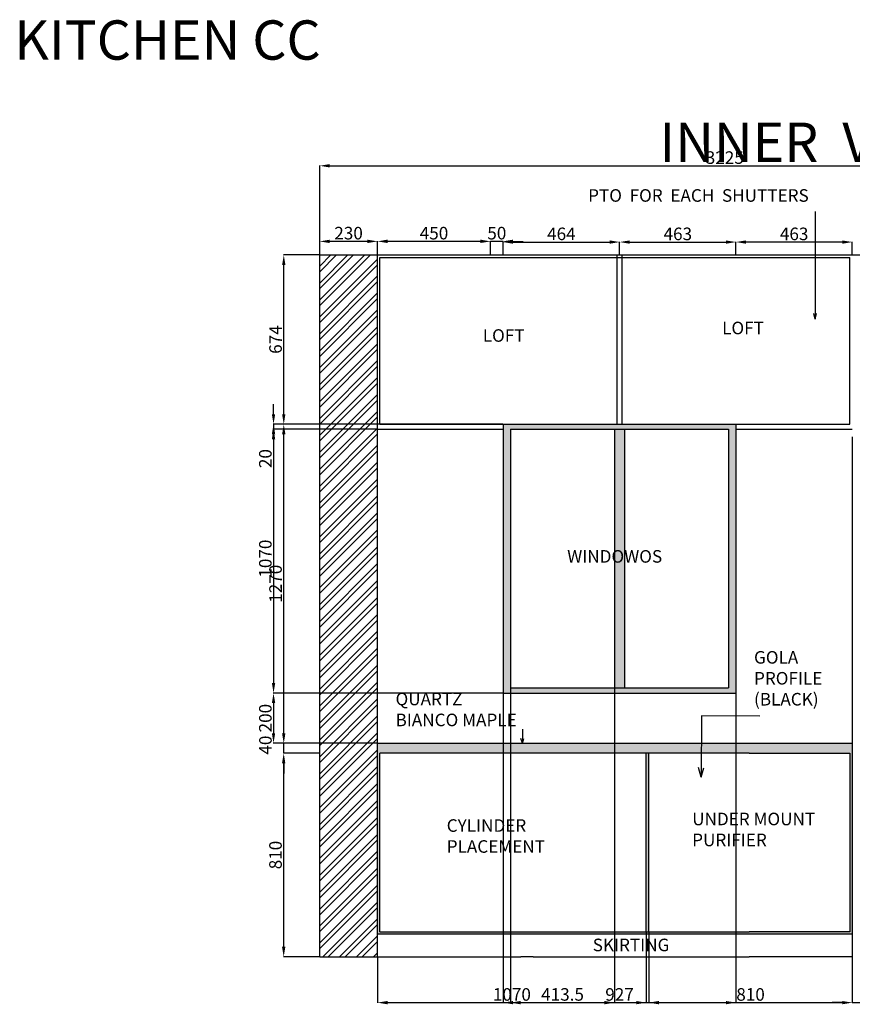
# Model space of a CAD drawing. Units: millimetres. Extents: x 144895 to 155057, y -2833 to 1092.
# Tile 3 of 4: x 148719 to 152033, y -2827 to 1092. Entities that reach past the tile are written whole.
import ezdxf

# ---------------------------------------------------------------- set-up
doc = ezdxf.new("R2010")
doc.units = ezdxf.units.MM
for name, color, linetype, lineweight in [('A-ANNO-DIMS', 2, 'Continuous', 18), ('A-ANNO-TEXT', 7, 'Continuous', 18), ('A-ELEV', 7, 'Continuous', 25), ('A-ELEV-PATT', 252, 'Continuous', 13), ('A-WALL-PATT', 8, 'Continuous', 13)]:
    doc.layers.add(name, color=color, linetype=linetype, lineweight=lineweight)
doc.styles.get("Standard").update_dxf_attribs({"font": 'arial.ttf'})
doc.dimstyles.new('ISO-25', dxfattribs={"dimtxt": 50, "dimasz": 40, "dimexe": 1.25, "dimexo": 0.625, "dimtad": 1, "dimtxsty": 'Standard', "dimcen": 2.5, "dimadec": 0, "dimazin": 0, "dimtfac": 1, "dimtmove": 0, "dimatfit": 3, "dimfxl": 1, "dimarcsym": 0})

# ---------------------------------------------------------------- blocks, each defined once
blk = doc.blocks.new('*D40')
at = {"layer": 'A-ANNO-DIMS', "color": 0, "lineweight": -2, "transparency": 16777216}
for p, q in [((149912.6, -1827.9), (149768.7, -1827.9)), ((149770, -2597.9), (149770, -1867.9)), ((149912.6, -2637.9), (149768.7, -2637.9))]:
    blk.add_line(p, q, dxfattribs=at)
at = {"layer": 'A-ANNO-DIMS', "color": 0, "transparency": 16777216}
for points in [[(149763.3, -1867.9), (149776.6, -1867.9), (149770, -1827.9)], [(149763.3, -2597.9), (149776.6, -2597.9), (149770, -2637.9)]]:
    blk.add_solid(points, dxfattribs=at)
at = {"layer": 'Defpoints', "color": 0, "transparency": 16777216}
for p in [(149770, -1827.9), (149913.2, -1827.9), (149913.2, -2637.9)]:
    blk.add_point(p, dxfattribs=at)
at = {"layer": 'A-ANNO-DIMS', "color": 0, "transparency": 16777216, "insert": (149743.8, -2232.9), "char_height": 50, "attachment_point": 5, "rotation": 90}
blk.add_mtext('810', dxfattribs=at)
blk = doc.blocks.new('*D32')
at = {"layer": 'A-ANNO-DIMS', "color": 0, "lineweight": -2, "transparency": 16777216}
for p, q in [((149770, -1747.9), (149770, -1707.9)), ((149912.6, -1787.9), (149768.7, -1787.9)), ((149770, -1827.9), (149770, -1787.9)), ((149912.6, -1827.9), (149768.7, -1827.9)), ((149770, -1867.9), (149770, -1907.9))]:
    blk.add_line(p, q, dxfattribs=at)
at = {"layer": 'A-ANNO-DIMS', "color": 0, "transparency": 16777216}
for points in [[(149763.3, -1747.9), (149776.6, -1747.9), (149770, -1787.9)], [(149763.3, -1867.9), (149776.6, -1867.9), (149770, -1827.9)]]:
    blk.add_solid(points, dxfattribs=at)
at = {"layer": 'Defpoints', "color": 0, "transparency": 16777216}
for p in [(149770, -1787.9), (149913.2, -1787.9), (149913.2, -1827.9)]:
    blk.add_point(p, dxfattribs=at)
at = {"layer": 'A-ANNO-DIMS', "color": 0, "transparency": 16777216, "insert": (149703.8, -1795.3), "char_height": 50, "attachment_point": 5, "rotation": 90}
blk.add_mtext('40', dxfattribs=at)
blk = doc.blocks.new('*D34')
at = {"layer": 'A-ANNO-DIMS', "color": 0, "lineweight": -2, "ltscale": 20, "transparency": 16777216}
for p, q in [((150143.2, 156.7), (150143.2, 211.4)), ((150553.2, 210.1), (150183.2, 210.1)), ((150593.2, 156.7), (150593.2, 211.4))]:
    blk.add_line(p, q, dxfattribs=at)
at = {"layer": 'A-ANNO-DIMS', "color": 0, "ltscale": 20, "transparency": 16777216}
for points in [[(150183.2, 216.8), (150183.2, 203.5), (150143.2, 210.1)], [(150553.2, 216.8), (150553.2, 203.5), (150593.2, 210.1)]]:
    blk.add_solid(points, dxfattribs=at)
at = {"layer": 'Defpoints', "color": 0, "ltscale": 20, "transparency": 16777216}
for p in [(150143.2, 210.1), (150143.2, 156.1), (150593.2, 156.1)]:
    blk.add_point(p, dxfattribs=at)
at = {"layer": 'A-ANNO-DIMS', "color": 0, "ltscale": 20, "transparency": 16777216, "insert": (150368.2, 236.3), "char_height": 50, "attachment_point": 5}
blk.add_mtext('450', dxfattribs=at)
blk = doc.blocks.new('*D35')
at = {"layer": 'A-ANNO-DIMS', "color": 0, "lineweight": -2, "ltscale": 20, "transparency": 16777216}
for p, q in [((150553.2, 210.1), (150513.2, 210.1)), ((150593.2, 156.7), (150593.2, 211.4)), ((150643.2, 210.1), (150593.2, 210.1)), ((150643.2, 156.7), (150643.2, 211.4)), ((150683.2, 210.1), (150723.2, 210.1))]:
    blk.add_line(p, q, dxfattribs=at)
at = {"layer": 'A-ANNO-DIMS', "color": 0, "ltscale": 20, "transparency": 16777216}
for points in [[(150553.2, 216.8), (150553.2, 203.5), (150593.2, 210.1)], [(150683.2, 216.8), (150683.2, 203.5), (150643.2, 210.1)]]:
    blk.add_solid(points, dxfattribs=at)
at = {"layer": 'Defpoints', "color": 0, "ltscale": 20, "transparency": 16777216}
for p in [(150593.2, 210.1), (150593.2, 156.1), (150643.2, 156.1)]:
    blk.add_point(p, dxfattribs=at)
at = {"layer": 'A-ANNO-DIMS', "color": 0, "ltscale": 20, "transparency": 16777216, "insert": (150618.2, 236.3), "char_height": 50, "attachment_point": 5}
blk.add_mtext('50', dxfattribs=at)
blk = doc.blocks.new('*D36')
at = {"layer": 'A-ANNO-DIMS', "color": 0, "lineweight": -2, "ltscale": 20, "transparency": 16777216}
for p, q in [((150643.2, 156.7), (150643.2, 208.4)), ((150683.2, 207.2), (151067.2, 207.2)), ((151107.2, 156.7), (151107.2, 208.4))]:
    blk.add_line(p, q, dxfattribs=at)
at = {"layer": 'A-ANNO-DIMS', "color": 0, "ltscale": 20, "transparency": 16777216}
for points in [[(150683.2, 213.9), (150683.2, 200.5), (150643.2, 207.2)], [(151067.2, 213.9), (151067.2, 200.5), (151107.2, 207.2)]]:
    blk.add_solid(points, dxfattribs=at)
at = {"layer": 'Defpoints', "color": 0, "ltscale": 20, "transparency": 16777216}
for p in [(151107.2, 207.2), (150643.2, 156.1), (151107.2, 156.1)]:
    blk.add_point(p, dxfattribs=at)
at = {"layer": 'A-ANNO-DIMS', "color": 0, "ltscale": 20, "transparency": 16777216, "insert": (150875.2, 233.4), "char_height": 50, "attachment_point": 5}
blk.add_mtext('464', dxfattribs=at)
blk = doc.blocks.new('*D37')
at = {"layer": 'A-ANNO-DIMS', "color": 0, "lineweight": -2, "ltscale": 20, "transparency": 16777216}
for p, q in [((151107.2, 156.7), (151107.2, 208.4)), ((151147.2, 207.2), (151530.2, 207.2)), ((151570.2, 156.7), (151570.2, 208.4))]:
    blk.add_line(p, q, dxfattribs=at)
at = {"layer": 'A-ANNO-DIMS', "color": 0, "ltscale": 20, "transparency": 16777216}
for points in [[(151147.2, 213.8), (151147.2, 200.5), (151107.2, 207.2)], [(151530.2, 213.8), (151530.2, 200.5), (151570.2, 207.2)]]:
    blk.add_solid(points, dxfattribs=at)
at = {"layer": 'Defpoints', "color": 0, "ltscale": 20, "transparency": 16777216}
for p in [(151570.2, 207.2), (151107.2, 156.1), (151570.2, 156.1)]:
    blk.add_point(p, dxfattribs=at)
at = {"layer": 'A-ANNO-DIMS', "color": 0, "ltscale": 20, "transparency": 16777216, "insert": (151338.7, 233.3), "char_height": 50, "attachment_point": 5}
blk.add_mtext('463', dxfattribs=at)
blk = doc.blocks.new('*D41')
at = {"layer": 'A-ANNO-DIMS', "color": 0, "lineweight": -2, "ltscale": 20, "transparency": 16777216}
for p, q in [((151570.2, 156.7), (151570.2, 208.4)), ((151993.2, 207.2), (151610.2, 207.2)), ((152033.2, 156.7), (152033.2, 208.4))]:
    blk.add_line(p, q, dxfattribs=at)
at = {"layer": 'A-ANNO-DIMS', "color": 0, "ltscale": 20, "transparency": 16777216}
for points in [[(151610.2, 213.8), (151610.2, 200.5), (151570.2, 207.2)], [(151993.2, 213.8), (151993.2, 200.5), (152033.2, 207.2)]]:
    blk.add_solid(points, dxfattribs=at)
at = {"layer": 'Defpoints', "color": 0, "ltscale": 20, "transparency": 16777216}
for p in [(151570.2, 207.2), (151570.2, 156.1), (152033.2, 156.1)]:
    blk.add_point(p, dxfattribs=at)
at = {"layer": 'A-ANNO-DIMS', "color": 0, "ltscale": 20, "transparency": 16777216, "insert": (151801.7, 233.3), "char_height": 50, "attachment_point": 5}
blk.add_mtext('463', dxfattribs=at)
blk = doc.blocks.new('*D42')
at = {"layer": 'A-ANNO-DIMS', "color": 0, "lineweight": -2, "ltscale": 20, "transparency": 16777216}
for p, q in [((149913.2, 156.7), (149913.2, 211.2)), ((150103.2, 210), (149953.2, 210)), ((150143.2, 156.7), (150143.2, 211.2))]:
    blk.add_line(p, q, dxfattribs=at)
at = {"layer": 'A-ANNO-DIMS', "color": 0, "ltscale": 20, "transparency": 16777216}
for points in [[(149953.2, 216.7), (149953.2, 203.3), (149913.2, 210)], [(150103.2, 216.7), (150103.2, 203.3), (150143.2, 210)]]:
    blk.add_solid(points, dxfattribs=at)
at = {"layer": 'Defpoints', "color": 0, "ltscale": 20, "transparency": 16777216}
for p in [(149913.2, 210), (149913.2, 156.1), (150143.2, 156.1)]:
    blk.add_point(p, dxfattribs=at)
at = {"layer": 'A-ANNO-DIMS', "color": 0, "ltscale": 20, "transparency": 16777216, "insert": (150028.2, 236.2), "char_height": 50, "attachment_point": 5}
blk.add_mtext('230', dxfattribs=at)
blk = doc.blocks.new('*D30')
at = {"layer": 'A-ANNO-DIMS', "color": 0, "lineweight": -2, "ltscale": 20, "transparency": 16777216}
for p, q in [((149912.6, -517.9), (149769, -517.9)), ((149770.3, -1747.9), (149770.3, -557.9)), ((149905.4, -1787.9), (149769, -1787.9))]:
    blk.add_line(p, q, dxfattribs=at)
at = {"layer": 'A-ANNO-DIMS', "color": 0, "ltscale": 20, "transparency": 16777216}
for points in [[(149763.6, -557.9), (149776.9, -557.9), (149770.3, -517.9)], [(149763.6, -1747.9), (149776.9, -1747.9), (149770.3, -1787.9)]]:
    blk.add_solid(points, dxfattribs=at)
at = {"layer": 'Defpoints', "color": 0, "ltscale": 20, "transparency": 16777216}
for p in [(149770.3, -517.9), (149913.2, -517.9), (149906, -1787.9)]:
    blk.add_point(p, dxfattribs=at)
at = {"layer": 'A-ANNO-DIMS', "color": 0, "ltscale": 20, "transparency": 16777216, "insert": (149744.1, -1152.9), "char_height": 50, "attachment_point": 5, "rotation": 90}
blk.add_mtext('1270', dxfattribs=at)
blk = doc.blocks.new('*D31')
at = {"layer": 'A-ANNO-DIMS', "color": 0, "lineweight": -2, "ltscale": 20, "transparency": 16777216}
for p, q in [((149912.6, 156.1), (149769, 156.1)), ((149770.3, -477.9), (149770.3, 116.1)), ((149912.6, -517.9), (149769, -517.9))]:
    blk.add_line(p, q, dxfattribs=at)
at = {"layer": 'A-ANNO-DIMS', "color": 0, "ltscale": 20, "transparency": 16777216}
for points in [[(149763.6, 116.1), (149776.9, 116.1), (149770.3, 156.1)], [(149763.6, -477.9), (149776.9, -477.9), (149770.3, -517.9)]]:
    blk.add_solid(points, dxfattribs=at)
at = {"layer": 'Defpoints', "color": 0, "ltscale": 20, "transparency": 16777216}
for p in [(149770.3, 156.1), (149913.2, 156.1), (149913.2, -517.9)]:
    blk.add_point(p, dxfattribs=at)
at = {"layer": 'A-ANNO-DIMS', "color": 0, "ltscale": 20, "transparency": 16777216, "insert": (149744.1, -180.9), "char_height": 50, "attachment_point": 5, "rotation": 90}
blk.add_mtext('674', dxfattribs=at)
blk = doc.blocks.new('*D59')
at = {"layer": 'A-ANNO-DIMS', "color": 0, "lineweight": -2, "ltscale": 20, "transparency": 16777216}
for p, q in [((149913.2, 156.7), (149913.2, 512.1)), ((149953.2, 510.8), (153098.2, 510.8)), ((153138.2, 156.7), (153138.2, 512.1))]:
    blk.add_line(p, q, dxfattribs=at)
at = {"layer": 'A-ANNO-DIMS', "color": 0, "ltscale": 20, "transparency": 16777216}
for points in [[(149953.2, 517.5), (149953.2, 504.2), (149913.2, 510.8)], [(153098.2, 517.5), (153098.2, 504.2), (153138.2, 510.8)]]:
    blk.add_solid(points, dxfattribs=at)
at = {"layer": 'Defpoints', "color": 0, "ltscale": 20, "transparency": 16777216}
for p in [(153138.2, 510.8), (149913.2, 156.1), (153138.2, 156.1)]:
    blk.add_point(p, dxfattribs=at)
at = {"layer": 'A-ANNO-DIMS', "color": 0, "ltscale": 20, "transparency": 16777216, "insert": (151525.7, 537), "char_height": 50, "attachment_point": 5}
blk.add_mtext('3225', dxfattribs=at)
blk = doc.blocks.new('*D61')
at = {"layer": 'A-ANNO-DIMS', "color": 0, "lineweight": -2, "ltscale": 20, "transparency": 16777216}
for p, q in [((151213.2, -2538.5), (151213.2, -2821.7)), ((150143.2, -2638.5), (150143.2, -2821.7)), ((150183.2, -2820.4), (151173.2, -2820.4))]:
    blk.add_line(p, q, dxfattribs=at)
at = {"layer": 'A-ANNO-DIMS', "color": 0, "ltscale": 20, "transparency": 16777216}
for points in [[(150183.2, -2813.8), (150183.2, -2827.1), (150143.2, -2820.4)], [(151173.2, -2813.8), (151173.2, -2827.1), (151213.2, -2820.4)]]:
    blk.add_solid(points, dxfattribs=at)
at = {"layer": 'Defpoints', "color": 0, "ltscale": 20, "transparency": 16777216}
for p in [(151213.2, -2537.9), (150143.2, -2637.9), (151213.2, -2820.4)]:
    blk.add_point(p, dxfattribs=at)
at = {"layer": 'A-ANNO-DIMS', "color": 0, "ltscale": 20, "transparency": 16777216, "insert": (150678.2, -2794.3), "char_height": 50, "attachment_point": 5}
blk.add_mtext('1070', dxfattribs=at)
blk = doc.blocks.new('*D62')
at = {"layer": 'A-ANNO-DIMS', "color": 0, "lineweight": -2, "ltscale": 20, "transparency": 16777216}
for p, q in [((151223.2, -2538.5), (151223.2, -2821.7)), ((152033.2, -2638.5), (152033.2, -2821.7)), ((151263.2, -2820.4), (151993.2, -2820.4))]:
    blk.add_line(p, q, dxfattribs=at)
at = {"layer": 'A-ANNO-DIMS', "color": 0, "ltscale": 20, "transparency": 16777216}
for points in [[(151263.2, -2813.8), (151263.2, -2827.1), (151223.2, -2820.4)], [(151993.2, -2813.8), (151993.2, -2827.1), (152033.2, -2820.4)]]:
    blk.add_solid(points, dxfattribs=at)
at = {"layer": 'Defpoints', "color": 0, "ltscale": 20, "transparency": 16777216}
for p in [(151223.2, -2537.9), (152033.2, -2637.9), (152033.2, -2820.4)]:
    blk.add_point(p, dxfattribs=at)
at = {"layer": 'A-ANNO-DIMS', "color": 0, "ltscale": 20, "transparency": 16777216, "insert": (151628.2, -2794.3), "char_height": 50, "attachment_point": 5}
blk.add_mtext('810', dxfattribs=at)
blk = doc.blocks.new('*D63')
at = {"layer": 'A-ANNO-DIMS', "color": 0, "lineweight": -2, "ltscale": 20, "transparency": 16777216}
for p, q in [((150643.2, -1588.5), (150643.2, -2821.7)), ((151570.2, -1588.5), (151570.2, -2821.7)), ((150683.2, -2820.4), (151530.2, -2820.4))]:
    blk.add_line(p, q, dxfattribs=at)
at = {"layer": 'A-ANNO-DIMS', "color": 0, "ltscale": 20, "transparency": 16777216}
for points in [[(150683.2, -2813.8), (150683.2, -2827.1), (150643.2, -2820.4)], [(151530.2, -2813.8), (151530.2, -2827.1), (151570.2, -2820.4)]]:
    blk.add_solid(points, dxfattribs=at)
at = {"layer": 'Defpoints', "color": 0, "ltscale": 20, "transparency": 16777216}
for p in [(150643.2, -1587.9), (151570.2, -1587.9), (151570.2, -2820.4)]:
    blk.add_point(p, dxfattribs=at)
at = {"layer": 'A-ANNO-DIMS', "color": 0, "ltscale": 20, "transparency": 16777216, "insert": (151106.7, -2794.3), "char_height": 50, "attachment_point": 5}
blk.add_mtext('927', dxfattribs=at)
blk = doc.blocks.new('*D64')
at = {"layer": 'A-ANNO-DIMS', "color": 0, "lineweight": -2, "ltscale": 20, "transparency": 16777216}
for p, q in [((150673.2, -1568.5), (150673.2, -2821.7)), ((151086.7, -1568.5), (151086.7, -2821.7)), ((150713.2, -2820.4), (151046.7, -2820.4))]:
    blk.add_line(p, q, dxfattribs=at)
at = {"layer": 'A-ANNO-DIMS', "color": 0, "ltscale": 20, "transparency": 16777216}
for points in [[(150713.2, -2813.8), (150713.2, -2827.1), (150673.2, -2820.4)], [(151046.7, -2813.8), (151046.7, -2827.1), (151086.7, -2820.4)]]:
    blk.add_solid(points, dxfattribs=at)
at = {"layer": 'Defpoints', "color": 0, "ltscale": 20, "transparency": 16777216}
for p in [(150673.2, -1567.9), (151086.7, -1567.9), (151086.7, -2820.4)]:
    blk.add_point(p, dxfattribs=at)
at = {"layer": 'A-ANNO-DIMS', "color": 0, "ltscale": 20, "transparency": 16777216, "insert": (150879.9, -2794.2), "char_height": 50, "attachment_point": 5}
blk.add_mtext('413.5', dxfattribs=at)
blk = doc.blocks.new('*D65')
at = {"layer": 'A-ANNO-DIMS', "color": 0, "lineweight": -2, "ltscale": 20, "transparency": 16777216}
for p, q in [((150642.6, -517.9), (149728.3, -517.9)), ((149729.5, -557.9), (149729.5, -1547.9)), ((150642.6, -1587.9), (149728.3, -1587.9))]:
    blk.add_line(p, q, dxfattribs=at)
at = {"layer": 'A-ANNO-DIMS', "color": 0, "ltscale": 20, "transparency": 16777216}
for points in [[(149722.9, -557.9), (149736.2, -557.9), (149729.5, -517.9)], [(149722.9, -1547.9), (149736.2, -1547.9), (149729.5, -1587.9)]]:
    blk.add_solid(points, dxfattribs=at)
at = {"layer": 'Defpoints', "color": 0, "ltscale": 20, "transparency": 16777216}
for p in [(150643.2, -517.9), (149729.5, -1587.9), (150643.2, -1587.9)]:
    blk.add_point(p, dxfattribs=at)
at = {"layer": 'A-ANNO-DIMS', "color": 0, "ltscale": 20, "transparency": 16777216, "insert": (149703.4, -1052.9), "char_height": 50, "attachment_point": 5, "rotation": 90}
blk.add_mtext('1070', dxfattribs=at)
blk = doc.blocks.new('*D66')
at = {"layer": 'A-ANNO-DIMS', "color": 0, "lineweight": -2, "ltscale": 20, "transparency": 16777216}
for p, q in [((150642.6, -1587.9), (149728.3, -1587.9)), ((149729.5, -1627.9), (149729.5, -1747.9)), ((150142.6, -1787.9), (149728.3, -1787.9))]:
    blk.add_line(p, q, dxfattribs=at)
at = {"layer": 'A-ANNO-DIMS', "color": 0, "ltscale": 20, "transparency": 16777216}
for points in [[(149722.9, -1627.9), (149736.2, -1627.9), (149729.5, -1587.9)], [(149722.9, -1747.9), (149736.2, -1747.9), (149729.5, -1787.9)]]:
    blk.add_solid(points, dxfattribs=at)
at = {"layer": 'Defpoints', "color": 0, "ltscale": 20, "transparency": 16777216}
for p in [(150643.2, -1587.9), (149729.5, -1787.9), (150143.2, -1787.9)]:
    blk.add_point(p, dxfattribs=at)
at = {"layer": 'A-ANNO-DIMS', "color": 0, "ltscale": 20, "transparency": 16777216, "insert": (149703.4, -1687.9), "char_height": 50, "attachment_point": 5, "rotation": 90}
blk.add_mtext('200', dxfattribs=at)
blk = doc.blocks.new('*D68')
at = {"layer": 'A-ANNO-DIMS', "color": 0, "lineweight": -2, "ltscale": 20, "transparency": 16777216}
for p, q in [((149729.5, -477.9), (149729.5, -437.9)), ((150152.6, -517.9), (149728.3, -517.9)), ((150142.6, -537.9), (149728.3, -537.9)), ((149729.5, -517.9), (149729.5, -537.9)), ((149729.5, -577.9), (149729.5, -691.5))]:
    blk.add_line(p, q, dxfattribs=at)
at = {"layer": 'A-ANNO-DIMS', "color": 0, "ltscale": 20, "transparency": 16777216}
for points in [[(149722.9, -477.9), (149736.2, -477.9), (149729.5, -517.9)], [(149722.9, -577.9), (149736.2, -577.9), (149729.5, -537.9)]]:
    blk.add_solid(points, dxfattribs=at)
at = {"layer": 'Defpoints', "color": 0, "ltscale": 20, "transparency": 16777216}
for p in [(149729.5, -537.9), (150143.2, -537.9), (150153.2, -517.9)]:
    blk.add_point(p, dxfattribs=at)
at = {"layer": 'A-ANNO-DIMS', "color": 0, "ltscale": 20, "transparency": 16777216, "insert": (149703.4, -654.7), "char_height": 50, "attachment_point": 5, "rotation": 90}
blk.add_mtext('20', dxfattribs=at)
blk = doc.blocks.new('*D70')
at = {"layer": 'A-ANNO-DIMS', "color": 0, "lineweight": -2, "ltscale": 20, "transparency": 16777216}
for p, q in [((152033.2, -568.5), (152033.2, -2821.7)), ((152083.2, -568.5), (152083.2, -2821.7)), ((151993.2, -2820.4), (151953.2, -2820.4)), ((152033.2, -2820.4), (152083.2, -2820.4)), ((152123.2, -2820.4), (152235.9, -2820.4))]:
    blk.add_line(p, q, dxfattribs=at)
at = {"layer": 'A-ANNO-DIMS', "color": 0, "ltscale": 20, "transparency": 16777216}
for points in [[(151993.2, -2813.8), (151993.2, -2827.1), (152033.2, -2820.4)], [(152123.2, -2813.8), (152123.2, -2827.1), (152083.2, -2820.4)]]:
    blk.add_solid(points, dxfattribs=at)
at = {"layer": 'Defpoints', "color": 0, "ltscale": 20, "transparency": 16777216}
for p in [(152033.2, -567.9), (152083.2, -567.9), (152083.2, -2820.4)]:
    blk.add_point(p, dxfattribs=at)
at = {"layer": 'A-ANNO-DIMS', "color": 0, "ltscale": 20, "transparency": 16777216, "insert": (152199.5, -2794.3), "char_height": 50, "attachment_point": 5}
blk.add_mtext('50', dxfattribs=at)

msp = doc.modelspace()

# ---------------------------------------------------------------- hatches: boundary and pattern name
at = {"layer": 'A-ELEV-PATT', "ltscale": 20}
h = msp.add_hatch(color=256, dxfattribs=at)
h.dxf.hatch_style = 1
h.paths.add_polyline_path([(150643.194, -1587.921), (151570.194, -1587.921), (151570.194, -517.921), (150643.194, -517.921)])
h.paths.add_polyline_path([(150673.194, -537.921), (151540.194, -537.921), (151540.194, -1567.921), (150673.194, -1567.921)], flags=16)
h.paths.add_polyline_path([(151086.694, -1567.921), (151126.694, -1567.921), (151126.694, -537.921), (151086.694, -537.921)], flags=16)
h.paths.add_polyline_path([(150885.127, -1097.22), (151317.528, -1097.22), (151317.528, -994.184), (150885.127, -994.184)], flags=8)
h = msp.add_hatch(color=256, dxfattribs=at)
h.dxf.hatch_style = 1
h.paths.add_polyline_path([(151223.194, -1827.921), (151213.194, -1827.921), (151213.194, -2537.921), (151223.194, -2537.921)], flags=17)
h.paths.add_polyline_path([(151432.009, -1787.921), (150143.194, -1787.921), (150143.194, -2547.921), (152033.194, -2547.921), (152033.194, -1787.921), (151432.009, -1787.921), (151431.804, -1827.921), (151623.194, -1827.921), (152023.194, -1827.921), (152023.194, -2537.921), (151623.194, -2537.921), (151213.194, -2537.921), (150153.194, -2537.921), (150153.194, -1827.921), (151213.194, -1827.921), (151223.194, -1827.921), (151431.804, -1827.921)])
h.paths.add_polyline_path([(150400.933, -2252.777), (150852.877, -2252.777), (150852.877, -2065.556), (150400.933, -2065.556)], flags=25)
at = {"layer": 'A-WALL-PATT'}
h = msp.add_hatch(dxfattribs=at)
h.set_pattern_fill('ANSI32', color=256, scale=5)
h.set_pattern_definition([(45, (4775.734, -17.217), (-33.67596, 33.67596), []), (45, (4798.185, -17.217), (-33.67596, 33.67596), [])])
h.paths.add_polyline_path([(149913.194, -1787.921), (149913.194, -2637.921), (150143.194, -2637.921), (150143.194, -1787.921), (150143.194, 156.079), (149913.194, 156.079), (149913.194, -517.921)])

# ---------------------------------------------------------------- linework, layer by layer
at = {"layer": 'A-ELEV', "ltscale": 20}
for p, q in [((151885.745, 328.326), (151885.745, -99.239)), ((151885.745, -99.239), (151880.068, -77.03)), ((151885.745, -99.239), (151891.181, -77.574)), ((150643.194, -517.921), (150643.194, -1587.921)), ((150673.194, -537.921), (150673.194, -1567.921)), ((151086.694, -537.921), (151086.694, -1567.921)), ((151126.694, -537.921), (151126.694, -1567.921)), ((151540.194, -537.921), (151540.194, -1567.921)), ((151570.194, -517.921), (151570.194, -1587.921)), ((151432.569, -1678.603), (151431.314, -1923.446)), ((151665.681, -1679.797), (151432.569, -1678.603)), ((150720.491, -1732.255), (150720.491, -1787.921)), ((150720.491, -1787.921), (150713.793, -1768.531)), ((150720.491, -1787.921), (150725.525, -1769)), ((151431.314, -1923.446), (151420.534, -1884.663)), ((151431.314, -1923.446), (151441.96, -1885.925)), ((150763.194, -2637.921), (150713.194, -2637.921))]:
    msp.add_line(p, q, dxfattribs=at)
at = {"layer": 'A-ELEV'}
for p, q in [((149913.194, 156.079), (153138.194, 156.079)), ((149913.194, -517.921), (149913.194, 156.079)), ((150143.194, -1787.921), (150143.194, 156.079)), ((150153.194, -517.921), (150153.194, 146.079)), ((150153.194, 146.079), (152023.194, 146.079)), ((151097.194, -517.921), (151097.194, 156.079)), ((151117.194, -517.921), (151117.194, 156.079)), ((152023.194, -517.921), (152023.194, 146.079)), ((149912.032, -537.921), (149913.194, -537.921)), ((149913.194, -1787.921), (149913.194, -517.921)), ((150143.194, -537.921), (150643.194, -537.921)), ((150153.194, -517.921), (152023.194, -517.921)), ((150673.194, -537.921), (151540.194, -537.921)), ((151570.194, -537.921), (152033.194, -537.921)), ((150643.194, -1587.921), (151570.194, -1587.921)), ((150673.194, -1567.921), (151540.194, -1567.921)), ((149913.194, -2637.921), (149913.194, -1787.921)), ((150143.194, -2637.921), (150143.194, -1787.921)), ((150143.194, -1787.921), (152033.194, -1787.921)), ((151213.194, -1827.921), (150153.194, -1827.921)), ((150153.194, -2537.921), (150153.194, -1827.921)), ((151213.194, -2537.921), (151213.194, -1827.921)), ((151623.194, -1827.921), (151213.194, -1827.921)), ((151223.194, -2537.921), (151223.194, -1827.921)), ((151623.194, -1827.921), (152023.194, -1827.921)), ((152023.194, -1827.921), (152023.194, -2537.921)), ((150153.194, -2537.921), (151213.194, -2537.921)), ((151213.194, -2537.921), (151623.194, -2537.921)), ((152023.194, -2537.921), (151623.194, -2537.921)), ((152033.194, -2547.921), (150143.194, -2547.921)), ((149913.194, -2637.921), (150713.194, -2637.921)), ((150763.194, -2637.921), (151213.194, -2637.921)), ((151213.194, -2637.921), (151623.194, -2637.921)), ((152033.194, -2637.921), (151623.194, -2637.921))]:
    msp.add_line(p, q, dxfattribs=at)

# ---------------------------------------------------------------- texts
at = {"layer": 'A-ANNO-TEXT', "attachment_point": 1}
for s, width, gutter_width, insert, char_height in [('KITCHEN CC', 9064.84564, 39.102, (148697.633, 1089.671), 156.408), ('INNER  VIEW', 9064.84564, 39.102, (151265.645, 682.915), 156.40804), ('PTO  FOR  EACH  SHUTTERS', 2897.81963, 12.5, (150981.654, 417.705), 50), ('LOFT ', 2897.81963, 12.5, (151515.077, -109.832), 50), ('LOFT ', 2897.81963, 12.5, (150562.435, -139.751), 50), ('WINDOWOS', 2897.81963, 12.5, (150898.48, -1019.031), 50), ('GOLA \\PPROFILE \\P(BLACK)', 2897.81963, 12.5, (151641.959, -1420.925), 50), ('QUARTZ\\PBIANCO MAPLE', 2897.81963, 12.5, (150215.141, -1586.687), 50), ('UNDER MOUNT \\PPURIFIER ', 2897.81963, 12.5, (151395.859, -2064.37), 50), ('\\pxi-2,l3,t3;CYLINDER\\PPLACEMENT', 2897.81963, 12.5, (150368.822, -2090.436), 50), ('SKIRTING', 2897.81963, 12.5, (150999.908, -2565.784), 50)]:
    msp.add_mtext_dynamic_manual_height_columns(s, width=width, gutter_width=gutter_width, heights=[0], dxfattribs=dict(at, insert=insert, char_height=char_height))

# ---------------------------------------------------------------- dimensions: what is measured, and where the dimension line sits
at = {"layer": 'A-ANNO-DIMS', "ltscale": 20}
for base, p1, p2, override, picture, middle in [((153138.194, 510.826), (149913.194, 156.079), (153138.194, 156.079), {"dimdec": 0, "dimlfac": 1, "dimrnd": 0, "dimzin": 0, "dimdsep": 46, "dimlunit": 2}, '*D59', (151525.694, 536.996)), ((149913.194, 209.993), (150143.194, 156.079), (149913.194, 156.079), {"dimclrd": 0, "dimclre": 0, "dimclrt": 0}, '*D42', (150028.194, 236.164)), ((150143.194, 210.129), (150593.194, 156.079), (150143.194, 156.079), {"dimclrd": 0, "dimclre": 0, "dimclrt": 0}, '*D34', (150368.194, 236.283)), ((151107.194, 207.198), (150643.194, 156.079), (151107.194, 156.079), {"dimclrd": 0, "dimclre": 0, "dimclrt": 0}, '*D36', (150875.194, 233.352)), ((151570.194, 207.163), (151107.194, 156.079), (151570.194, 156.079), {"dimclrd": 0, "dimclre": 0, "dimclrt": 0}, '*D37', (151338.694, 233.334)), ((151570.194, 207.163), (152033.194, 156.079), (151570.194, 156.079), {"dimclrd": 0, "dimclre": 0, "dimclrt": 0}, '*D41', (151801.694, 233.334)), ((152083.194, -2820.421), (152033.194, -567.921), (152083.194, -567.921), {"dimdec": 0, "dimlfac": 1, "dimrnd": 0, "dimzin": 0, "dimdsep": 46, "dimlunit": 2}, '*D70', (152199.546, -2794.267)), ((151570.194, -2820.421), (150643.194, -1587.921), (151570.194, -1587.921), {"dimdec": 0, "dimlfac": 1, "dimrnd": 0, "dimzin": 0, "dimdsep": 46, "dimlunit": 2}, '*D63', (151106.694, -2794.267)), ((151086.694, -2820.421), (150673.194, -1567.921), (151086.694, -1567.921), {"dimdec": 1, "dimlfac": 1, "dimrnd": 0, "dimzin": 0, "dimdsep": 46, "dimlunit": 2}, '*D64', (150879.944, -2794.25)), ((151213.194, -2820.421), (150143.194, -2637.921), (151213.194, -2537.921), {"dimdec": 0, "dimlfac": 1, "dimrnd": 0, "dimzin": 0, "dimdsep": 46, "dimlunit": 2}, '*D61', (150678.194, -2794.267)), ((152033.194, -2820.421), (151223.194, -2537.921), (152033.194, -2637.921), {"dimdec": 0, "dimlfac": 1, "dimrnd": 0, "dimzin": 0, "dimdsep": 46, "dimlunit": 2}, '*D62', (151628.194, -2794.267))]:
    dim = msp.add_linear_dim(base=base, p1=p1, p2=p2, dimstyle='ISO-25', override=override, dxfattribs=at)
    dim.commit()
    dim.dimension.update_dxf_attribs({"geometry": picture, "text_midpoint": middle})
dim = msp.add_linear_dim(base=(150593.194, 210.129), p1=(150643.194, 156.079), p2=(150593.194, 156.079), dimstyle='ISO-25', override={"dimclrd": 0, "dimclre": 0, "dimclrt": 0}, dxfattribs=at)
dim.commit()
dim.dimension.update_dxf_attribs({"geometry": '*D35', "text_midpoint": (150618.194, 210.129), "dimtype": 160})
for base, p1, p2, override, picture, middle in [((149770.262, 156.079), (149913.194, -517.921), (149913.194, 156.079), {"dimclrd": 0, "dimclre": 0, "dimclrt": 0}, '*D31', (149744.109, -180.921)), ((149729.532, -537.921), (150153.194, -517.921), (150143.194, -537.921), {"dimdec": 0, "dimlfac": 1, "dimrnd": 0, "dimzin": 0, "dimdsep": 46, "dimlunit": 2}, '*D68', (149703.378, -654.698)), ((149729.532, -1587.921), (150643.194, -517.921), (150643.194, -1587.921), {"dimdec": 0, "dimlfac": 1, "dimrnd": 0, "dimzin": 0, "dimdsep": 46, "dimlunit": 2}, '*D65', (149703.378, -1052.921)), ((149770.262, -517.921), (149906.002, -1787.921), (149913.194, -517.921), {"dimclrd": 0, "dimclre": 0, "dimclrt": 0}, '*D30', (149744.109, -1152.921)), ((149729.532, -1787.921), (150643.194, -1587.921), (150143.194, -1787.921), {"dimdec": 0, "dimlfac": 1, "dimrnd": 0, "dimzin": 0, "dimdsep": 46, "dimlunit": 2}, '*D66', (149703.378, -1687.921))]:
    dim = msp.add_linear_dim(base=base, p1=p1, p2=p2, angle=90, dimstyle='ISO-25', override=override, dxfattribs=at)
    dim.commit()
    dim.dimension.update_dxf_attribs({"geometry": picture, "text_midpoint": middle})
at = {"layer": 'A-ANNO-DIMS'}
for base, p1, p2, override, picture, middle in [((149769.979, -1787.921), (149913.194, -1827.921), (149913.194, -1787.921), {"dimclrd": 0, "dimclre": 0, "dimclrt": 0, "dimtmove": 1}, '*D32', (149703.826, -1795.296)), ((149769.979, -1827.921), (149913.194, -2637.921), (149913.194, -1827.921), {"dimclrd": 0, "dimclre": 0, "dimclrt": 0}, '*D40', (149743.826, -2232.921))]:
    dim = msp.add_linear_dim(base=base, p1=p1, p2=p2, angle=90, dimstyle='ISO-25', override=override, dxfattribs=at)
    dim.commit()
    dim.dimension.update_dxf_attribs({"geometry": picture, "text_midpoint": middle})

doc.saveas('drawing.dxf')
